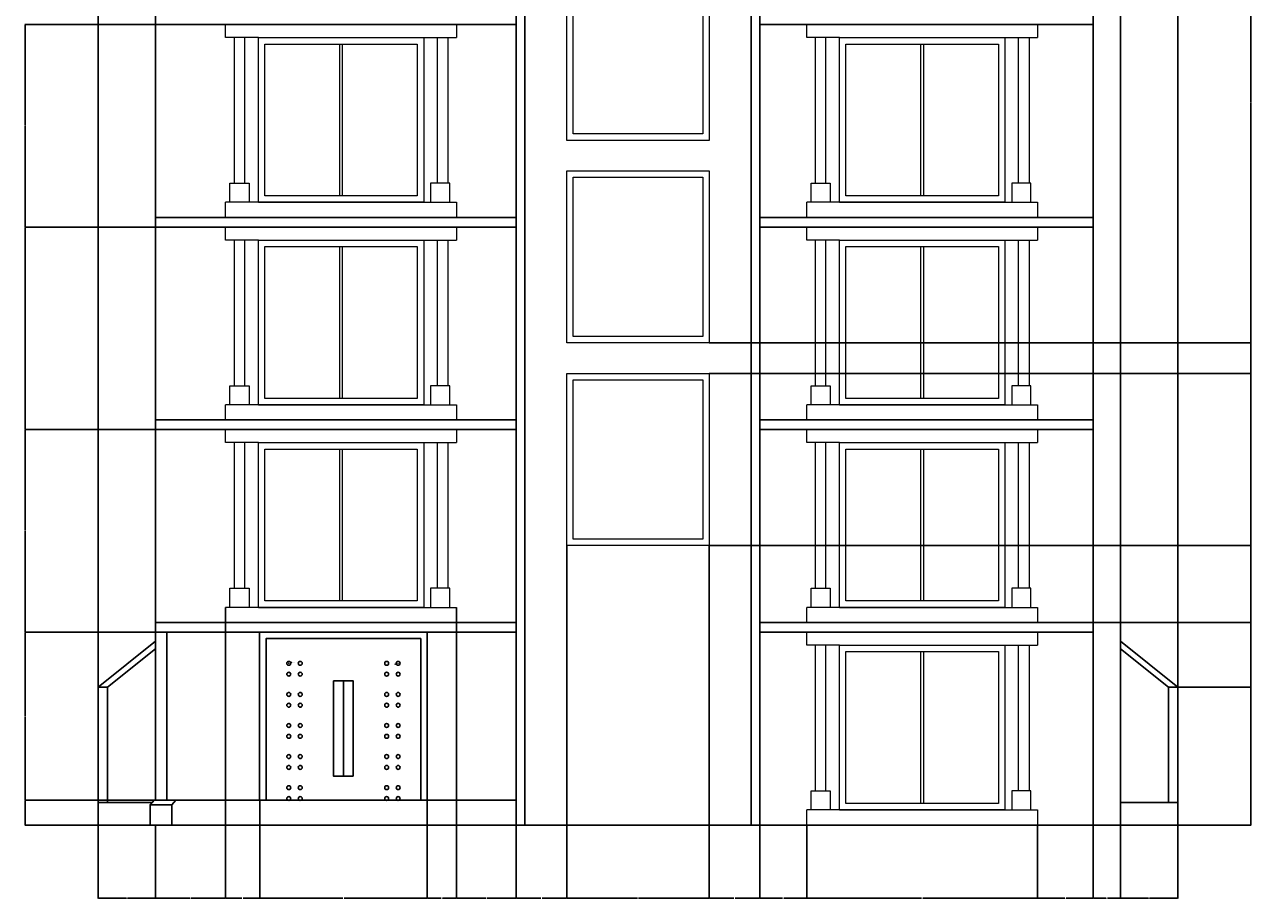
# Model space of a CAD drawing. Units: inches. Extents: x 3024 to 4744, y 1110 to 2100.
# Tile 28 of 29: x 3980 to 4744, y 1110 to 1654. Entities that reach past the tile are written whole.
import ezdxf

# ---------------------------------------------------------------- set-up
doc = ezdxf.new("R2010")
doc.units = ezdxf.units.IN
for name, color, linetype, lineweight in [('A-ANNO-DIMS', 2, 'Continuous', 18), ('A-ELEV', 7, 'Continuous', 25), ('A-GLAZ', 4, 'Continuous', 18)]:
    doc.layers.add(name, color=color, linetype=linetype, lineweight=lineweight)
doc.styles.get("Standard").update_dxf_attribs({"font": 'arial.ttf'})
doc.dimstyles.get("Standard").update_dxf_attribs({"dimtxt": 0.18, "dimasz": 0.18, "dimexe": 0.18, "dimexo": 0.0625, "dimgap": 0.09, "dimtad": 0, "dimtih": 1, "dimtoh": 1, "dimdec": 1, "dimzin": 0, "dimdsep": 46, "dimlunit": 3, "dimtxsty": 'Standard', "dimcen": 0.09, "dimadec": 0, "dimazin": 0, "dimtfac": 1, "dimtdec": 1, "dimtofl": 0, "dimtmove": 0, "dimatfit": 3, "dimfxl": 1, "dimtolj": 1, "dimtzin": 0, "dimarcsym": 0})

# ---------------------------------------------------------------- blocks, each defined once
blk = doc.blocks.new('WIN-BALCONY-B')
for p, q in [((4125.9, 1897.49), (4105.47, 1897.49)), ((4125.9, 1897.49), (4249.1, 1897.49)), ((4125.9, 1795.04), (4105.47, 1795.04)), ((4125.9, 1795.04), (4249.1, 1795.04))]:
    blk.add_line(p, q)
for points in [[(4105.47, 1897.49), (4105.47, 1905.61), (4249.1, 1905.61), (4249.1, 1897.49)], [(4249.1, 1795.04), (4249.1, 1785.61), (4105.47, 1785.61), (4105.47, 1795.04)]]:
    blk.add_lwpolyline(points)
for points in [[(4110.83, 1806.87), (4117.36, 1806.87), (4117.36, 1897.49), (4110.83, 1897.49)], [(4228.68, 1795.04), (4125.9, 1795.04), (4125.9, 1897.49), (4228.68, 1897.49)], [(4224.68, 1799.04), (4129.9, 1799.04), (4129.9, 1893.49), (4224.68, 1893.49)], [(4176.55, 1893.49), (4178.02, 1893.49), (4178.02, 1799.04), (4176.55, 1799.04)], [(4243.74, 1806.87), (4237.21, 1806.87), (4237.21, 1897.49), (4243.74, 1897.49)], [(4120.03, 1795.04), (4108.16, 1795.04), (4108.16, 1806.87), (4120.03, 1806.87)], [(4233.01, 1795.04), (4244.87, 1795.04), (4244.87, 1806.87), (4233.01, 1806.87)]]:
    blk.add_lwpolyline(points, close=True)
blk = doc.blocks.new('WIN-CENTRE-PLAIN')
for points in [[(4317.72, 1940.61), (4406.22, 1940.61), (4406.22, 1833.52), (4317.72, 1833.52)], [(4321.72, 1936.61), (4402.22, 1936.61), (4402.22, 1837.52), (4321.72, 1837.52)]]:
    blk.add_lwpolyline(points, close=True)
blk = doc.blocks.new('*D16')
at = {"layer": 'A-ANNO-DIMS', "color": 0, "lineweight": -2, "transparency": 16777216}
for p, q in [((4026.29, 1155.55), (4026.29, 1109.93)), ((4061.97, 1155.55), (4061.97, 1109.93)), ((4026.47, 1110.11), (4043.74, 1110.11)), ((4061.79, 1110.11), (4044.53, 1110.11))]:
    blk.add_line(p, q, dxfattribs=at)
at = {"layer": 'A-ANNO-DIMS', "color": 0, "transparency": 16777216}
for points in [[(4026.47, 1110.14), (4026.47, 1110.08), (4026.29, 1110.11)], [(4061.79, 1110.14), (4061.79, 1110.08), (4061.97, 1110.11)]]:
    blk.add_solid(points, dxfattribs=at)
at = {"layer": 'Defpoints', "color": 0, "transparency": 16777216}
for p in [(4026.29, 1155.61), (4061.97, 1155.61), (4061.97, 1110.11)]:
    blk.add_point(p, dxfattribs=at)
at = {"layer": 'A-ANNO-DIMS', "color": 0, "transparency": 16777216, "insert": (4044.13, 1110.11), "char_height": 0.18, "attachment_point": 5}
blk.add_mtext('\\A1;35.68', dxfattribs=at)
blk = doc.blocks.new('*D17')
at = {"layer": 'A-ANNO-DIMS', "color": 0, "lineweight": -2, "transparency": 16777216}
for p, q in [((4105.47, 1290.98), (4105.47, 1109.93)), ((4061.97, 1155.55), (4061.97, 1109.93)), ((4062.15, 1110.11), (4083.39, 1110.11)), ((4105.29, 1110.11), (4084.05, 1110.11))]:
    blk.add_line(p, q, dxfattribs=at)
at = {"layer": 'A-ANNO-DIMS', "color": 0, "transparency": 16777216}
for points in [[(4062.15, 1110.14), (4062.15, 1110.08), (4061.97, 1110.11)], [(4105.29, 1110.14), (4105.29, 1110.08), (4105.47, 1110.11)]]:
    blk.add_solid(points, dxfattribs=at)
at = {"layer": 'Defpoints', "color": 0, "transparency": 16777216}
for p in [(4105.47, 1291.04), (4061.97, 1155.61), (4105.47, 1110.11)]:
    blk.add_point(p, dxfattribs=at)
at = {"layer": 'A-ANNO-DIMS', "color": 0, "transparency": 16777216, "insert": (4083.72, 1110.11), "char_height": 0.18, "attachment_point": 5}
blk.add_mtext('\\A1;43.5', dxfattribs=at)
blk = doc.blocks.new('*D18')
at = {"layer": 'A-ANNO-DIMS', "color": 0, "lineweight": -2, "transparency": 16777216}
for p, q in [((4105.47, 1290.98), (4105.47, 1109.93)), ((4126.66, 1170.96), (4126.66, 1109.93)), ((4105.65, 1110.11), (4115.67, 1110.11)), ((4126.48, 1110.11), (4116.46, 1110.11))]:
    blk.add_line(p, q, dxfattribs=at)
at = {"layer": 'A-ANNO-DIMS', "color": 0, "transparency": 16777216}
for points in [[(4105.65, 1110.14), (4105.65, 1110.08), (4105.47, 1110.11)], [(4126.48, 1110.14), (4126.48, 1110.08), (4126.66, 1110.11)]]:
    blk.add_solid(points, dxfattribs=at)
at = {"layer": 'Defpoints', "color": 0, "transparency": 16777216}
for p in [(4105.47, 1291.04), (4126.66, 1171.02), (4126.66, 1110.11)]:
    blk.add_point(p, dxfattribs=at)
at = {"layer": 'A-ANNO-DIMS', "color": 0, "transparency": 16777216, "insert": (4116.06, 1110.11), "char_height": 0.18, "attachment_point": 5}
blk.add_mtext('\\A1;21.19', dxfattribs=at)
blk = doc.blocks.new('*D19')
at = {"layer": 'A-ANNO-DIMS', "color": 0, "lineweight": -2, "transparency": 16777216}
for p, q in [((4126.66, 1170.96), (4126.66, 1109.93)), ((4230.89, 1170.96), (4230.89, 1109.93)), ((4126.84, 1110.11), (4178.32, 1110.11)), ((4230.71, 1110.11), (4179.23, 1110.11))]:
    blk.add_line(p, q, dxfattribs=at)
at = {"layer": 'A-ANNO-DIMS', "color": 0, "transparency": 16777216}
for points in [[(4126.84, 1110.14), (4126.84, 1110.08), (4126.66, 1110.11)], [(4230.71, 1110.14), (4230.71, 1110.08), (4230.89, 1110.11)]]:
    blk.add_solid(points, dxfattribs=at)
at = {"layer": 'Defpoints', "color": 0, "transparency": 16777216}
for p in [(4126.66, 1171.02), (4230.89, 1171.02), (4230.89, 1110.11)]:
    blk.add_point(p, dxfattribs=at)
at = {"layer": 'A-ANNO-DIMS', "color": 0, "transparency": 16777216, "insert": (4178.77, 1110.11), "char_height": 0.18, "attachment_point": 5}
blk.add_mtext('\\A1;104.23', dxfattribs=at)
blk = doc.blocks.new('*D20')
at = {"layer": 'A-ANNO-DIMS', "color": 0, "lineweight": -2, "transparency": 16777216}
for p, q in [((4249.1, 1290.98), (4249.1, 1109.93)), ((4230.89, 1170.96), (4230.89, 1109.93)), ((4231.07, 1110.11), (4239.54, 1110.11)), ((4248.92, 1110.11), (4240.45, 1110.11))]:
    blk.add_line(p, q, dxfattribs=at)
at = {"layer": 'A-ANNO-DIMS', "color": 0, "transparency": 16777216}
for points in [[(4231.07, 1110.14), (4231.07, 1110.08), (4230.89, 1110.11)], [(4248.92, 1110.14), (4248.92, 1110.08), (4249.1, 1110.11)]]:
    blk.add_solid(points, dxfattribs=at)
at = {"layer": 'Defpoints', "color": 0, "transparency": 16777216}
for p in [(4249.1, 1291.04), (4230.89, 1171.02), (4249.1, 1110.11)]:
    blk.add_point(p, dxfattribs=at)
at = {"layer": 'A-ANNO-DIMS', "color": 0, "transparency": 16777216, "insert": (4240, 1110.11), "char_height": 0.18, "attachment_point": 5}
blk.add_mtext('\\A1;18.217', dxfattribs=at)
blk = doc.blocks.new('*D21')
at = {"layer": 'A-ANNO-DIMS', "color": 0, "lineweight": -2, "transparency": 16777216}
for p, q in [((4249.1, 1290.98), (4249.1, 1109.93)), ((4286.2, 1155.55), (4286.2, 1109.93)), ((4249.28, 1110.11), (4267.35, 1110.11)), ((4286.02, 1110.11), (4267.96, 1110.11))]:
    blk.add_line(p, q, dxfattribs=at)
at = {"layer": 'A-ANNO-DIMS', "color": 0, "transparency": 16777216}
for points in [[(4249.28, 1110.14), (4249.28, 1110.08), (4249.1, 1110.11)], [(4286.02, 1110.14), (4286.02, 1110.08), (4286.2, 1110.11)]]:
    blk.add_solid(points, dxfattribs=at)
at = {"layer": 'Defpoints', "color": 0, "transparency": 16777216}
for p in [(4249.1, 1291.04), (4286.2, 1155.61), (4286.2, 1110.11)]:
    blk.add_point(p, dxfattribs=at)
at = {"layer": 'A-ANNO-DIMS', "color": 0, "transparency": 16777216, "insert": (4267.65, 1110.11), "char_height": 0.18, "attachment_point": 5}
blk.add_mtext('\\A1;37.1', dxfattribs=at)
blk = doc.blocks.new('*D22')
at = {"layer": 'A-ANNO-DIMS', "color": 0, "lineweight": -2, "transparency": 16777216}
for p, q in [((4317.72, 1329.46), (4317.72, 1109.93)), ((4286.2, 1155.55), (4286.2, 1109.93)), ((4286.38, 1110.11), (4301.57, 1110.11)), ((4317.54, 1110.11), (4302.36, 1110.11))]:
    blk.add_line(p, q, dxfattribs=at)
at = {"layer": 'A-ANNO-DIMS', "color": 0, "transparency": 16777216}
for points in [[(4286.38, 1110.14), (4286.38, 1110.08), (4286.2, 1110.11)], [(4317.54, 1110.14), (4317.54, 1110.08), (4317.72, 1110.11)]]:
    blk.add_solid(points, dxfattribs=at)
at = {"layer": 'Defpoints', "color": 0, "transparency": 16777216}
for p in [(4317.72, 1329.52), (4286.2, 1155.61), (4317.72, 1110.11)]:
    blk.add_point(p, dxfattribs=at)
at = {"layer": 'A-ANNO-DIMS', "color": 0, "transparency": 16777216, "insert": (4301.96, 1110.11), "char_height": 0.18, "attachment_point": 5}
blk.add_mtext('\\A1;31.52', dxfattribs=at)
blk = doc.blocks.new('*D23')
at = {"layer": 'A-ANNO-DIMS', "color": 0, "lineweight": -2, "transparency": 16777216}
for p, q in [((4317.72, 1329.46), (4317.72, 1109.93)), ((4406.22, 1329.46), (4406.22, 1109.93)), ((4317.9, 1110.11), (4361.65, 1110.11)), ((4406.04, 1110.11), (4362.3, 1110.11))]:
    blk.add_line(p, q, dxfattribs=at)
at = {"layer": 'A-ANNO-DIMS', "color": 0, "transparency": 16777216}
for points in [[(4317.9, 1110.14), (4317.9, 1110.08), (4317.72, 1110.11)], [(4406.04, 1110.14), (4406.04, 1110.08), (4406.22, 1110.11)]]:
    blk.add_solid(points, dxfattribs=at)
at = {"layer": 'Defpoints', "color": 0, "transparency": 16777216}
for p in [(4317.72, 1329.52), (4406.22, 1329.52), (4406.22, 1110.11)]:
    blk.add_point(p, dxfattribs=at)
at = {"layer": 'A-ANNO-DIMS', "color": 0, "transparency": 16777216, "insert": (4361.97, 1110.11), "char_height": 0.18, "attachment_point": 5}
blk.add_mtext('\\A1;88.5', dxfattribs=at)
blk = doc.blocks.new('*D24')
at = {"layer": 'A-ANNO-DIMS', "color": 0, "lineweight": -2, "transparency": 16777216}
for p, q in [((4406.22, 1329.46), (4406.22, 1109.93)), ((4437.74, 1155.55), (4437.74, 1109.93)), ((4406.4, 1110.11), (4421.59, 1110.11)), ((4437.56, 1110.11), (4422.37, 1110.11))]:
    blk.add_line(p, q, dxfattribs=at)
at = {"layer": 'A-ANNO-DIMS', "color": 0, "transparency": 16777216}
for points in [[(4406.4, 1110.14), (4406.4, 1110.08), (4406.22, 1110.11)], [(4437.56, 1110.14), (4437.56, 1110.08), (4437.74, 1110.11)]]:
    blk.add_solid(points, dxfattribs=at)
at = {"layer": 'Defpoints', "color": 0, "transparency": 16777216}
for p in [(4406.22, 1329.52), (4437.74, 1155.61), (4437.74, 1110.11)]:
    blk.add_point(p, dxfattribs=at)
at = {"layer": 'A-ANNO-DIMS', "color": 0, "transparency": 16777216, "insert": (4421.98, 1110.11), "char_height": 0.18, "attachment_point": 5}
blk.add_mtext('\\A1;31.52', dxfattribs=at)
blk = doc.blocks.new('*D25')
at = {"layer": 'A-ANNO-DIMS', "color": 0, "lineweight": -2, "transparency": 16777216}
for p, q in [((4437.74, 1155.55), (4437.74, 1109.93)), ((4466.9, 1155.55), (4466.9, 1109.93)), ((4437.92, 1110.11), (4451.92, 1110.11)), ((4466.72, 1110.11), (4452.72, 1110.11))]:
    blk.add_line(p, q, dxfattribs=at)
at = {"layer": 'A-ANNO-DIMS', "color": 0, "transparency": 16777216}
for points in [[(4437.92, 1110.14), (4437.92, 1110.08), (4437.74, 1110.11)], [(4466.72, 1110.14), (4466.72, 1110.08), (4466.9, 1110.11)]]:
    blk.add_solid(points, dxfattribs=at)
at = {"layer": 'Defpoints', "color": 0, "transparency": 16777216}
for p in [(4437.74, 1155.61), (4466.9, 1155.61), (4466.9, 1110.11)]:
    blk.add_point(p, dxfattribs=at)
at = {"layer": 'A-ANNO-DIMS', "color": 0, "transparency": 16777216, "insert": (4452.32, 1110.11), "char_height": 0.18, "attachment_point": 5}
blk.add_mtext('\\A1;29.16', dxfattribs=at)
blk = doc.blocks.new('*D26')
at = {"layer": 'A-ANNO-DIMS', "color": 0, "lineweight": -2, "transparency": 16777216}
for p, q in [((4466.9, 1155.55), (4466.9, 1109.93)), ((4610.54, 1155.55), (4610.54, 1109.93)), ((4467.08, 1110.11), (4538.26, 1110.11)), ((4610.36, 1110.11), (4539.17, 1110.11))]:
    blk.add_line(p, q, dxfattribs=at)
at = {"layer": 'A-ANNO-DIMS', "color": 0, "transparency": 16777216}
for points in [[(4467.08, 1110.14), (4467.08, 1110.08), (4466.9, 1110.11)], [(4610.36, 1110.14), (4610.36, 1110.08), (4610.54, 1110.11)]]:
    blk.add_solid(points, dxfattribs=at)
at = {"layer": 'Defpoints', "color": 0, "transparency": 16777216}
for p in [(4466.9, 1155.61), (4610.54, 1155.61), (4610.54, 1110.11)]:
    blk.add_point(p, dxfattribs=at)
at = {"layer": 'A-ANNO-DIMS', "color": 0, "transparency": 16777216, "insert": (4538.72, 1110.11), "char_height": 0.18, "attachment_point": 5}
blk.add_mtext('\\A1;143.64', dxfattribs=at)
blk = doc.blocks.new('*D27')
at = {"layer": 'A-ANNO-DIMS', "color": 0, "lineweight": -2, "transparency": 16777216}
for p, q in [((4610.54, 1155.55), (4610.54, 1109.93)), ((4645.06, 1155.55), (4645.06, 1109.93)), ((4610.72, 1110.11), (4627.4, 1110.11)), ((4644.88, 1110.11), (4628.19, 1110.11))]:
    blk.add_line(p, q, dxfattribs=at)
at = {"layer": 'A-ANNO-DIMS', "color": 0, "transparency": 16777216}
for points in [[(4610.72, 1110.14), (4610.72, 1110.08), (4610.54, 1110.11)], [(4644.88, 1110.14), (4644.88, 1110.08), (4645.06, 1110.11)]]:
    blk.add_solid(points, dxfattribs=at)
at = {"layer": 'Defpoints', "color": 0, "transparency": 16777216}
for p in [(4610.54, 1155.61), (4645.06, 1155.61), (4645.06, 1110.11)]:
    blk.add_point(p, dxfattribs=at)
at = {"layer": 'A-ANNO-DIMS', "color": 0, "transparency": 16777216, "insert": (4627.8, 1110.11), "char_height": 0.18, "attachment_point": 5}
blk.add_mtext('\\A1;34.52', dxfattribs=at)
blk = doc.blocks.new('*D28')
at = {"layer": 'A-ANNO-DIMS', "color": 0, "lineweight": -2, "transparency": 16777216}
for p, q in [((4645.06, 1155.55), (4645.06, 1109.93)), ((4661.97, 1155.55), (4661.97, 1109.93)), ((4645.24, 1110.11), (4653.06, 1110.11)), ((4661.79, 1110.11), (4653.97, 1110.11))]:
    blk.add_line(p, q, dxfattribs=at)
at = {"layer": 'A-ANNO-DIMS', "color": 0, "transparency": 16777216}
for points in [[(4645.24, 1110.14), (4645.24, 1110.08), (4645.06, 1110.11)], [(4661.79, 1110.14), (4661.79, 1110.08), (4661.97, 1110.11)]]:
    blk.add_solid(points, dxfattribs=at)
at = {"layer": 'Defpoints', "color": 0, "transparency": 16777216}
for p in [(4645.06, 1155.61), (4661.97, 1155.61), (4661.97, 1110.11)]:
    blk.add_point(p, dxfattribs=at)
at = {"layer": 'A-ANNO-DIMS', "color": 0, "transparency": 16777216, "insert": (4653.51, 1110.11), "char_height": 0.18, "attachment_point": 5}
blk.add_mtext('\\A1;16.913', dxfattribs=at)
blk = doc.blocks.new('*D29')
at = {"layer": 'A-ANNO-DIMS', "color": 0, "lineweight": -2, "transparency": 16777216}
for p, q in [((4661.97, 1155.55), (4661.97, 1109.93)), ((4697.65, 1155.55), (4697.65, 1109.93)), ((4662.15, 1110.11), (4679.42, 1110.11)), ((4697.47, 1110.11), (4680.2, 1110.11))]:
    blk.add_line(p, q, dxfattribs=at)
at = {"layer": 'A-ANNO-DIMS', "color": 0, "transparency": 16777216}
for points in [[(4662.15, 1110.14), (4662.15, 1110.08), (4661.97, 1110.11)], [(4697.47, 1110.14), (4697.47, 1110.08), (4697.65, 1110.11)]]:
    blk.add_solid(points, dxfattribs=at)
at = {"layer": 'Defpoints', "color": 0, "transparency": 16777216}
for p in [(4661.97, 1155.61), (4697.65, 1155.61), (4697.65, 1110.11)]:
    blk.add_point(p, dxfattribs=at)
at = {"layer": 'A-ANNO-DIMS', "color": 0, "transparency": 16777216, "insert": (4679.81, 1110.11), "char_height": 0.18, "attachment_point": 5}
blk.add_mtext('\\A1;35.68', dxfattribs=at)
blk = doc.blocks.new('*D30')
at = {"layer": 'A-ANNO-DIMS', "color": 0, "lineweight": -2, "transparency": 16777216}
for p, q in [((4026.29, 1241.5), (4026.29, 2100.44)), ((4026.47, 2100.26), (4038.86, 2100.26)), ((4052.03, 2100.26), (4039.65, 2100.26)), ((4052.21, 1911.67), (4052.21, 2100.44))]:
    blk.add_line(p, q, dxfattribs=at)
at = {"layer": 'A-ANNO-DIMS', "color": 0, "transparency": 16777216}
for points in [[(4026.47, 2100.29), (4026.47, 2100.23), (4026.29, 2100.26)], [(4052.03, 2100.29), (4052.03, 2100.23), (4052.21, 2100.26)]]:
    blk.add_solid(points, dxfattribs=at)
at = {"layer": 'Defpoints', "color": 0, "transparency": 16777216}
for p in [(4052.21, 2100.26), (4052.21, 1911.61), (4026.29, 1241.43)]:
    blk.add_point(p, dxfattribs=at)
at = {"layer": 'A-ANNO-DIMS', "color": 0, "transparency": 16777216, "insert": (4039.25, 2100.26), "char_height": 0.18, "attachment_point": 5}
blk.add_mtext('\\A1;25.92', dxfattribs=at)
blk = doc.blocks.new('*D34')
at = {"layer": 'A-ANNO-DIMS', "color": 0, "lineweight": -2, "transparency": 16777216}
for p, q in [((4671.73, 1911.67), (4671.73, 2100.44)), ((4671.91, 2100.26), (4684.29, 2100.26)), ((4697.47, 2100.26), (4685.08, 2100.26)), ((4697.65, 1241.5), (4697.65, 2100.44))]:
    blk.add_line(p, q, dxfattribs=at)
at = {"layer": 'A-ANNO-DIMS', "color": 0, "transparency": 16777216}
for points in [[(4671.91, 2100.29), (4671.91, 2100.23), (4671.73, 2100.26)], [(4697.47, 2100.29), (4697.47, 2100.23), (4697.65, 2100.26)]]:
    blk.add_solid(points, dxfattribs=at)
at = {"layer": 'Defpoints', "color": 0, "transparency": 16777216}
for p in [(4697.65, 2100.26), (4671.73, 1911.61), (4697.65, 1241.43)]:
    blk.add_point(p, dxfattribs=at)
at = {"layer": 'A-ANNO-DIMS', "color": 0, "transparency": 16777216, "insert": (4684.69, 2100.26), "char_height": 0.18, "attachment_point": 5}
blk.add_mtext('\\A1;25.92', dxfattribs=at)
blk = doc.blocks.new('*D35')
at = {"layer": 'A-ANNO-DIMS', "color": 0, "lineweight": -2, "transparency": 16777216}
for p, q in [((4061.91, 1171.02), (3980.61, 1171.02)), ((3980.79, 1170.84), (3980.79, 1163.5)), ((3980.79, 1155.79), (3980.79, 1163.14)), ((4061.91, 1155.61), (3980.61, 1155.61))]:
    blk.add_line(p, q, dxfattribs=at)
at = {"layer": 'A-ANNO-DIMS', "color": 0, "transparency": 16777216}
for points in [[(3980.76, 1170.84), (3980.82, 1170.84), (3980.79, 1171.02)], [(3980.76, 1155.79), (3980.82, 1155.79), (3980.79, 1155.61)]]:
    blk.add_solid(points, dxfattribs=at)
at = {"layer": 'Defpoints', "color": 0, "transparency": 16777216}
for p in [(3980.79, 1171.02), (4061.97, 1171.02), (4061.97, 1155.61)]:
    blk.add_point(p, dxfattribs=at)
at = {"layer": 'A-ANNO-DIMS', "color": 0, "transparency": 16777216, "insert": (3980.79, 1163.32), "char_height": 0.18, "attachment_point": 5}
blk.add_mtext('\\A1;15.413', dxfattribs=at)
blk = doc.blocks.new('*D36')
at = {"layer": 'A-ANNO-DIMS', "color": 0, "lineweight": -2, "transparency": 16777216}
for p, q in [((4061.91, 1275.61), (3980.61, 1275.61)), ((3980.79, 1275.43), (3980.79, 1223.5)), ((3980.79, 1171.2), (3980.79, 1223.14)), ((4061.91, 1171.02), (3980.61, 1171.02))]:
    blk.add_line(p, q, dxfattribs=at)
at = {"layer": 'A-ANNO-DIMS', "color": 0, "transparency": 16777216}
for points in [[(3980.76, 1275.43), (3980.82, 1275.43), (3980.79, 1275.61)], [(3980.76, 1171.2), (3980.82, 1171.2), (3980.79, 1171.02)]]:
    blk.add_solid(points, dxfattribs=at)
at = {"layer": 'Defpoints', "color": 0, "transparency": 16777216}
for p in [(3980.79, 1275.61), (4061.97, 1275.61), (4061.97, 1171.02)]:
    blk.add_point(p, dxfattribs=at)
at = {"layer": 'A-ANNO-DIMS', "color": 0, "transparency": 16777216, "insert": (3980.79, 1223.32), "char_height": 0.18, "attachment_point": 5}
blk.add_mtext('\\A1;104.59', dxfattribs=at)
blk = doc.blocks.new('*D37')
at = {"layer": 'A-ANNO-DIMS', "color": 0, "lineweight": -2, "transparency": 16777216}
for p, q in [((4061.91, 1401.61), (3980.61, 1401.61)), ((3980.79, 1401.43), (3980.79, 1338.79)), ((3980.79, 1275.79), (3980.79, 1338.43)), ((4061.91, 1275.61), (3980.61, 1275.61))]:
    blk.add_line(p, q, dxfattribs=at)
at = {"layer": 'A-ANNO-DIMS', "color": 0, "transparency": 16777216}
for points in [[(3980.76, 1401.43), (3980.82, 1401.43), (3980.79, 1401.61)], [(3980.76, 1275.79), (3980.82, 1275.79), (3980.79, 1275.61)]]:
    blk.add_solid(points, dxfattribs=at)
at = {"layer": 'Defpoints', "color": 0, "transparency": 16777216}
for p in [(3980.79, 1401.61), (4061.97, 1401.61), (4061.97, 1275.61)]:
    blk.add_point(p, dxfattribs=at)
at = {"layer": 'A-ANNO-DIMS', "color": 0, "transparency": 16777216, "insert": (3980.79, 1338.61), "char_height": 0.18, "attachment_point": 5}
blk.add_mtext('\\A1;126', dxfattribs=at)
blk = doc.blocks.new('*D38')
at = {"layer": 'A-ANNO-DIMS', "color": 0, "lineweight": -2, "transparency": 16777216}
for p, q in [((4061.91, 1527.61), (3980.61, 1527.61)), ((3980.79, 1527.43), (3980.79, 1464.79)), ((3980.79, 1401.79), (3980.79, 1464.43)), ((4061.91, 1401.61), (3980.61, 1401.61))]:
    blk.add_line(p, q, dxfattribs=at)
at = {"layer": 'A-ANNO-DIMS', "color": 0, "transparency": 16777216}
for points in [[(3980.76, 1527.43), (3980.82, 1527.43), (3980.79, 1527.61)], [(3980.76, 1401.79), (3980.82, 1401.79), (3980.79, 1401.61)]]:
    blk.add_solid(points, dxfattribs=at)
at = {"layer": 'Defpoints', "color": 0, "transparency": 16777216}
for p in [(3980.79, 1527.61), (4061.97, 1527.61), (4061.97, 1401.61)]:
    blk.add_point(p, dxfattribs=at)
at = {"layer": 'A-ANNO-DIMS', "color": 0, "transparency": 16777216, "insert": (3980.79, 1464.61), "char_height": 0.18, "attachment_point": 5}
blk.add_mtext('\\A1;126', dxfattribs=at)
blk = doc.blocks.new('*D39')
at = {"layer": 'A-ANNO-DIMS', "color": 0, "lineweight": -2, "transparency": 16777216}
for p, q in [((4061.91, 1653.61), (3980.61, 1653.61)), ((3980.79, 1653.43), (3980.79, 1590.79)), ((3980.79, 1527.79), (3980.79, 1590.43)), ((4061.91, 1527.61), (3980.61, 1527.61))]:
    blk.add_line(p, q, dxfattribs=at)
at = {"layer": 'A-ANNO-DIMS', "color": 0, "transparency": 16777216}
for points in [[(3980.76, 1653.43), (3980.82, 1653.43), (3980.79, 1653.61)], [(3980.76, 1527.79), (3980.82, 1527.79), (3980.79, 1527.61)]]:
    blk.add_solid(points, dxfattribs=at)
at = {"layer": 'Defpoints', "color": 0, "transparency": 16777216}
for p in [(3980.79, 1653.61), (4061.97, 1653.61), (4061.97, 1527.61)]:
    blk.add_point(p, dxfattribs=at)
at = {"layer": 'A-ANNO-DIMS', "color": 0, "transparency": 16777216, "insert": (3980.79, 1590.61), "char_height": 0.18, "attachment_point": 5}
blk.add_mtext('\\A1;126', dxfattribs=at)
blk = doc.blocks.new('*D45')
at = {"layer": 'A-ANNO-DIMS', "color": 0, "lineweight": -2, "transparency": 16777216}
for p, q in [((4697.71, 1241.43), (4743.33, 1241.43)), ((4743.15, 1241.25), (4743.15, 1198.7)), ((4743.15, 1155.79), (4743.15, 1198.34)), ((4697.71, 1155.61), (4743.33, 1155.61))]:
    blk.add_line(p, q, dxfattribs=at)
at = {"layer": 'A-ANNO-DIMS', "color": 0, "transparency": 16777216}
for points in [[(4743.12, 1241.25), (4743.18, 1241.25), (4743.15, 1241.43)], [(4743.12, 1155.79), (4743.18, 1155.79), (4743.15, 1155.61)]]:
    blk.add_solid(points, dxfattribs=at)
at = {"layer": 'Defpoints', "color": 0, "transparency": 16777216}
for p in [(4697.65, 1241.43), (4743.15, 1241.43), (4697.65, 1155.61)]:
    blk.add_point(p, dxfattribs=at)
at = {"layer": 'A-ANNO-DIMS', "color": 0, "transparency": 16777216, "insert": (4743.15, 1198.52), "char_height": 0.18, "attachment_point": 5}
blk.add_mtext('\\A1;85.82', dxfattribs=at)
blk = doc.blocks.new('*D46')
at = {"layer": 'A-ANNO-DIMS', "color": 0, "lineweight": -2, "transparency": 16777216}
for p, q in [((4406.28, 1329.52), (4743.33, 1329.52)), ((4743.15, 1329.34), (4743.15, 1305.75)), ((4743.15, 1281.79), (4743.15, 1305.39)), ((4645.12, 1281.61), (4743.33, 1281.61))]:
    blk.add_line(p, q, dxfattribs=at)
at = {"layer": 'A-ANNO-DIMS', "color": 0, "transparency": 16777216}
for points in [[(4743.12, 1329.34), (4743.18, 1329.34), (4743.15, 1329.52)], [(4743.12, 1281.79), (4743.18, 1281.79), (4743.15, 1281.61)]]:
    blk.add_solid(points, dxfattribs=at)
at = {"layer": 'Defpoints', "color": 0, "transparency": 16777216}
for p in [(4406.22, 1329.52), (4743.15, 1329.52), (4645.06, 1281.61)]:
    blk.add_point(p, dxfattribs=at)
at = {"layer": 'A-ANNO-DIMS', "color": 0, "transparency": 16777216, "insert": (4743.15, 1305.57), "char_height": 0.18, "attachment_point": 5}
blk.add_mtext('\\A1;47.91', dxfattribs=at)
blk = doc.blocks.new('*D47')
at = {"layer": 'A-ANNO-DIMS', "color": 0, "lineweight": -2, "transparency": 16777216}
for p, q in [((4406.28, 1455.52), (4743.33, 1455.52)), ((4743.15, 1455.34), (4743.15, 1446.25)), ((4743.15, 1436.79), (4743.15, 1445.88)), ((4406.28, 1436.61), (4743.33, 1436.61))]:
    blk.add_line(p, q, dxfattribs=at)
at = {"layer": 'A-ANNO-DIMS', "color": 0, "transparency": 16777216}
for points in [[(4743.12, 1455.34), (4743.18, 1455.34), (4743.15, 1455.52)], [(4743.12, 1436.79), (4743.18, 1436.79), (4743.15, 1436.61)]]:
    blk.add_solid(points, dxfattribs=at)
at = {"layer": 'Defpoints', "color": 0, "transparency": 16777216}
for p in [(4406.22, 1455.52), (4743.15, 1455.52), (4406.22, 1436.61)]:
    blk.add_point(p, dxfattribs=at)
at = {"layer": 'A-ANNO-DIMS', "color": 0, "transparency": 16777216, "insert": (4743.15, 1446.07), "char_height": 0.18, "attachment_point": 5}
blk.add_mtext('\\A1;18.92', dxfattribs=at)
blk = doc.blocks.new('*D76')
at = {"layer": 'A-ANNO-DIMS', "color": 0, "lineweight": -2, "transparency": 16777216}
for p, q in [((4144.67, 1256.23), (4144.85, 1256.23)), ((4144.76, 1256.14), (4144.76, 1256.32)), ((4146.57, 1256.89), (4146.06, 1256.71)), ((4146.75, 1256.89), (4146.57, 1256.89))]:
    blk.add_line(p, q, dxfattribs=at)
at = {"layer": 'A-ANNO-DIMS', "color": 0, "transparency": 16777216}
blk.add_solid([(4146.05, 1256.73), (4146.07, 1256.68), (4145.89, 1256.64)], dxfattribs=at)
at = {"layer": 'Defpoints', "color": 0, "transparency": 16777216}
for p in [(4143.62, 1255.81), (4145.89, 1256.64)]:
    blk.add_point(p, dxfattribs=at)
at = {"layer": 'A-ANNO-DIMS', "color": 0, "transparency": 16777216, "insert": (4147.5, 1256.89), "char_height": 0.18, "attachment_point": 5}
blk.add_mtext('\\A1;40X ∅2.414', dxfattribs=at)
blk = doc.blocks.new('*D78')
at = {"layer": 'A-ANNO-DIMS', "color": 0, "lineweight": -2, "transparency": 16777216}
for p, q in [((4448.39, 2054.76), (4743.33, 2054.76)), ((4743.15, 2054.58), (4743.15, 1605.37)), ((4743.15, 1155.79), (4743.15, 1605)), ((4697.71, 1155.61), (4743.33, 1155.61))]:
    blk.add_line(p, q, dxfattribs=at)
at = {"layer": 'A-ANNO-DIMS', "color": 0, "transparency": 16777216}
for points in [[(4743.12, 2054.58), (4743.18, 2054.58), (4743.15, 2054.76)], [(4743.12, 1155.79), (4743.18, 1155.79), (4743.15, 1155.61)]]:
    blk.add_solid(points, dxfattribs=at)
at = {"layer": 'Defpoints', "color": 0, "transparency": 16777216}
for p in [(4448.33, 2054.76), (4743.15, 2054.76), (4697.65, 1155.61)]:
    blk.add_point(p, dxfattribs=at)
at = {"layer": 'A-ANNO-DIMS', "color": 0, "transparency": 16777216, "insert": (4743.15, 1605.18), "char_height": 0.18, "attachment_point": 5}
blk.add_mtext('\\A1;899.15', dxfattribs=at)
blk = doc.blocks.new('*D130')
at = {"layer": 'A-ANNO-DIMS', "color": 0, "lineweight": -2, "transparency": 16777216}
for p, q in [((4210.76, 1255.66), (4210.94, 1255.66)), ((4210.94, 1255.66), (4211.46, 1255.82)), ((4212.7, 1256.23), (4212.88, 1256.23)), ((4212.79, 1256.14), (4212.79, 1256.32))]:
    blk.add_line(p, q, dxfattribs=at)
at = {"layer": 'A-ANNO-DIMS', "color": 0, "transparency": 16777216}
blk.add_solid([(4211.46, 1255.85), (4211.47, 1255.79), (4211.64, 1255.87)], dxfattribs=at)
at = {"layer": 'Defpoints', "color": 0, "transparency": 16777216}
for p in [(4211.64, 1255.87), (4213.94, 1256.59)]:
    blk.add_point(p, dxfattribs=at)
at = {"layer": 'A-ANNO-DIMS', "color": 0, "transparency": 16777216, "insert": (4210.01, 1255.66), "char_height": 0.18, "attachment_point": 5}
blk.add_mtext('\\A1;40X ∅2.414', dxfattribs=at)

msp = doc.modelspace()

# ---------------------------------------------------------------- linework, layer by layer
at = {"layer": 'A-ELEV'}
for p, q in [((4661.9711, 1155.6112), (4661.9711, 1911.6112)), ((4061.9711, 1171.0239), (4061.9711, 1905.6112)), ((4286.2022, 1653.6112), (4061.9711, 1653.6112)), ((4645.0576, 1653.6112), (4437.74, 1653.6112)), ((4061.9711, 1533.6112), (4286.2022, 1533.6112)), ((4286.2022, 1527.6112), (4061.9711, 1527.6112)), ((4437.74, 1533.6112), (4645.0576, 1533.6112)), ((4645.0576, 1527.6112), (4437.74, 1527.6112)), ((4061.9711, 1407.6112), (4286.2022, 1407.6112)), ((4437.74, 1407.6112), (4645.0576, 1407.6112)), ((4286.2022, 1401.6112), (4061.9711, 1401.6112)), ((4645.0576, 1401.6112), (4437.74, 1401.6112)), ((4061.9711, 1275.6112), (4061.9711, 1281.6112)), ((4061.9711, 1281.6112), (4286.2022, 1281.6112)), ((4286.2022, 1275.6112), (4061.9711, 1275.6112)), ((4437.74, 1281.6112), (4645.0576, 1281.6112)), ((4645.0576, 1275.6112), (4437.74, 1275.6112)), ((4026.2926, 1241.4341), (4061.9711, 1269.9091)), ((4697.6496, 1241.4341), (4661.9711, 1269.9091)), ((4032.0358, 1241.4341), (4061.9711, 1265.3254)), ((4691.9063, 1241.4341), (4661.9711, 1265.3254)), ((4178.7732, 1245.2708), (4178.7732, 1185.9515)), ((4026.2926, 1155.6112), (4026.2926, 1169.5534)), ((4059.7347, 1169.5534), (4026.2926, 1169.5534)), ((4058.4636, 1168.0828), (4061.0058, 1171.0239)), ((4058.4636, 1168.0828), (4072.0743, 1168.0828)), ((4061.0058, 1171.0239), (4074.6165, 1171.0239)), ((4072.0743, 1168.0828), (4074.6165, 1171.0239)), ((4074.6165, 1171.0239), (4286.2022, 1171.0239)), ((4661.9711, 1169.5534), (4697.6496, 1169.5534)), ((4697.6496, 1155.6112), (4697.6496, 1169.5534)), ((4061.9711, 1155.6112), (4026.2926, 1155.6112)), ((4061.9711, 1155.6112), (4661.9711, 1155.6112)), ((4661.9711, 1155.6112), (4697.6496, 1155.6112))]:
    msp.add_line(p, q, dxfattribs=at)
for points in [[(4437.74, 1155.6112), (4286.2022, 1155.6112), (4286.2022, 2043.5286), (4437.74, 2043.5286)], [(4286.2022, 2043.5286), (4291.6033, 2043.5286), (4291.6033, 1155.6112), (4286.2022, 1155.6112)], [(4432.3389, 2043.5286), (4437.74, 2043.5286), (4437.74, 1155.6112), (4432.3389, 1155.6112)], [(4184.8844, 1185.9515), (4172.6619, 1185.9515), (4172.6619, 1245.2708), (4184.8844, 1245.2708)], [(4026.2926, 1169.5534), (4032.0358, 1169.5534), (4032.0358, 1241.4341), (4026.2926, 1241.4341)], [(4697.6496, 1169.5534), (4691.9063, 1169.5534), (4691.9063, 1241.4341), (4697.6496, 1241.4341)]]:
    msp.add_lwpolyline(points, close=True, dxfattribs=at)
for points in [[(4661.9711, 1155.6112), (4645.0576, 1155.6112), (4645.0576, 2009.1664)], [(4061.9711, 1275.6112), (4068.8827, 1275.6112), (4068.8827, 1171.0239)], [(4126.6597, 1171.0239), (4126.6597, 1275.6112), (4230.8866, 1275.6112), (4230.8866, 1171.0239)], [(4130.6597, 1171.0239), (4130.6597, 1271.6112), (4226.8866, 1271.6112), (4226.8866, 1171.0239)], [(4072.0743, 1155.6112), (4072.0743, 1168.0828), (4058.4636, 1168.0828), (4058.4636, 1155.6112)], [(4230.8866, 1155.6112), (4126.6597, 1155.6112)]]:
    msp.add_lwpolyline(points, dxfattribs=at)
for centre in [(4144.7575, 1256.2276), (4151.9042, 1256.2276), (4205.6422, 1256.2276), (4212.7888, 1256.2276), (4144.7575, 1249.4899), (4151.9042, 1249.4899), (4205.6422, 1249.4899), (4212.7888, 1249.4899), (4144.7575, 1236.8869), (4151.9042, 1236.8869), (4205.6422, 1236.8869), (4212.7888, 1236.8869), (4144.7575, 1230.1493), (4151.9042, 1230.1493), (4205.6422, 1230.1493), (4212.7888, 1230.1493), (4144.7575, 1217.5463), (4151.9042, 1217.5463), (4205.6422, 1217.5463), (4212.7888, 1217.5463), (4144.7575, 1210.8086), (4151.9042, 1210.8086), (4205.6422, 1210.8086), (4212.7888, 1210.8086), (4144.7575, 1198.2057), (4151.9042, 1198.2057), (4205.6422, 1198.2057), (4212.7888, 1198.2057), (4144.7575, 1191.468), (4151.9042, 1191.468), (4205.6422, 1191.468), (4212.7888, 1191.468), (4144.7575, 1178.8651), (4151.9042, 1178.8651), (4205.6422, 1178.8651), (4212.7888, 1178.8651), (4144.7575, 1172.1274), (4151.9042, 1172.1274), (4205.6422, 1172.1274), (4212.7888, 1172.1274)]:
    msp.add_circle(centre, 1.2071, dxfattribs=at)

# ---------------------------------------------------------------- block references
at = {"layer": 'A-GLAZ'}
for name, p in [('WIN-CENTRE-PLAIN', (0, -252)), ('WIN-BALCONY-B', (0, -252)), ('WIN-BALCONY-B', (361.4319, -252)), ('WIN-CENTRE-PLAIN', (0, -378)), ('WIN-BALCONY-B', (0, -378)), ('WIN-BALCONY-B', (361.4319, -378)), ('WIN-CENTRE-PLAIN', (0, -504)), ('WIN-BALCONY-B', (0, -504)), ('WIN-BALCONY-B', (361.4319, -504)), ('WIN-BALCONY-B', (361.4319, -630))]:
    msp.add_blockref(name, p, dxfattribs=at)

# ---------------------------------------------------------------- dimensions: what is measured, and where the dimension line sits
at = {"layer": 'A-ANNO-DIMS'}
for base, p1, p2, override, picture, middle in [((4052.2147, 2100.2584), (4026.2926, 1241.4341), (4052.2147, 1911.6112), {"dimdec": 2, "dimlfac": 1, "dimrnd": 0, "dimzin": 0, "dimdsep": 46, "dimlunit": 2}, '*D30', (4039.2536, 2100.2584)), ((4697.6496, 2100.2584), (4671.7274, 1911.6112), (4697.6496, 1241.4341), {"dimdec": 2, "dimlfac": 1, "dimrnd": 0, "dimzin": 0, "dimdsep": 46, "dimlunit": 2}, '*D34', (4684.6885, 2100.2584)), ((4317.7231, 1110.1112), (4286.2022, 1155.6112), (4317.7231, 1329.5246), {"dimdec": 2, "dimlfac": 1, "dimrnd": 0, "dimzin": 0, "dimdsep": 46, "dimlunit": 2}, '*D22', (4301.9626, 1110.1112)), ((4406.2191, 1110.1112), (4317.7231, 1329.5246), (4406.2191, 1329.5246), {"dimdec": 1, "dimlfac": 1, "dimrnd": 0, "dimzin": 0, "dimdsep": 46, "dimlunit": 2}, '*D23', (4361.9711, 1110.1112)), ((4437.74, 1110.1112), (4406.2191, 1329.5246), (4437.74, 1155.6112), {"dimdec": 2, "dimlfac": 1, "dimrnd": 0, "dimzin": 0, "dimdsep": 46, "dimlunit": 2}, '*D24', (4421.9795, 1110.1112)), ((4105.4683, 1110.1112), (4061.9711, 1155.6112), (4105.4683, 1291.0431), {"dimdec": 1, "dimlfac": 1, "dimrnd": 0, "dimzin": 0, "dimdsep": 46, "dimlunit": 2}, '*D17', (4083.7197, 1110.1112)), ((4126.6597, 1110.1112), (4105.4683, 1291.0431), (4126.6597, 1171.0239), {"dimdec": 2, "dimlfac": 1, "dimrnd": 0, "dimzin": 0, "dimdsep": 46, "dimlunit": 2}, '*D18', (4116.064, 1110.1112)), ((4249.104, 1110.1112), (4230.8866, 1171.0239), (4249.104, 1291.0431), {"dimdec": 3, "dimlfac": 1, "dimrnd": 0, "dimzin": 0, "dimdsep": 46, "dimlunit": 2}, '*D20', (4239.9953, 1110.1112)), ((4286.2022, 1110.1112), (4249.104, 1291.0431), (4286.2022, 1155.6112), {"dimdec": 1, "dimlfac": 1, "dimrnd": 0, "dimzin": 0, "dimdsep": 46, "dimlunit": 2}, '*D21', (4267.6531, 1110.1112)), ((4230.8866, 1110.1112), (4126.6597, 1171.0239), (4230.8866, 1171.0239), {"dimdec": 2, "dimlfac": 1, "dimrnd": 0, "dimzin": 0, "dimdsep": 46, "dimlunit": 2}, '*D19', (4178.7732, 1110.1112)), ((4061.9711, 1110.1112), (4026.2926, 1155.6112), (4061.9711, 1155.6112), {"dimdec": 2, "dimlfac": 1, "dimrnd": 0, "dimzin": 0, "dimdsep": 46, "dimlunit": 2}, '*D16', (4044.1318, 1110.1112)), ((4466.9002, 1110.1112), (4437.74, 1155.6112), (4466.9002, 1155.6112), {"dimdec": 2, "dimlfac": 1, "dimrnd": 0, "dimzin": 0, "dimdsep": 46, "dimlunit": 2}, '*D25', (4452.3201, 1110.1112)), ((4610.5359, 1110.1112), (4466.9002, 1155.6112), (4610.5359, 1155.6112), {"dimdec": 2, "dimlfac": 1, "dimrnd": 0, "dimzin": 0, "dimdsep": 46, "dimlunit": 2}, '*D26', (4538.718, 1110.1112)), ((4645.0576, 1110.1112), (4610.5359, 1155.6112), (4645.0576, 1155.6112), {"dimdec": 2, "dimlfac": 1, "dimrnd": 0, "dimzin": 0, "dimdsep": 46, "dimlunit": 2}, '*D27', (4627.7968, 1110.1112)), ((4661.97108, 1110.11117), (4645.05764, 1155.61117), (4661.97108, 1155.61117), {"dimdec": 3, "dimlfac": 1, "dimrnd": 0, "dimzin": 0, "dimdsep": 46, "dimlunit": 2}, '*D28', (4653.51436, 1110.11117)), ((4697.6496, 1110.1112), (4661.9711, 1155.6112), (4697.6496, 1155.6112), {"dimdec": 2, "dimlfac": 1, "dimrnd": 0, "dimzin": 0, "dimdsep": 46, "dimlunit": 2}, '*D29', (4679.8103, 1110.1112))]:
    dim = msp.add_linear_dim(base=base, p1=p1, p2=p2, dimstyle='Standard', override=override, dxfattribs=at)
    dim.commit()
    dim.dimension.update_dxf_attribs({"geometry": picture, "text_midpoint": middle})
for base, p1, p2, override, picture, middle in [((4743.1496, 2054.7584), (4697.6496, 1155.6112), (4448.326, 2054.7584), {"dimdec": 2, "dimlfac": 1, "dimrnd": 0, "dimzin": 0, "dimdsep": 46, "dimlunit": 2}, '*D78', (4743.1496, 1605.1848)), ((3980.7926, 1653.6112), (4061.9711, 1527.6112), (4061.9711, 1653.6112), {"dimdec": 0, "dimlfac": 1, "dimrnd": 0, "dimzin": 0, "dimdsep": 46, "dimlunit": 2}, '*D39', (3980.7926, 1590.6112)), ((3980.7926, 1527.6112), (4061.9711, 1401.6112), (4061.9711, 1527.6112), {"dimdec": 0, "dimlfac": 1, "dimrnd": 0, "dimzin": 0, "dimdsep": 46, "dimlunit": 2}, '*D38', (3980.7926, 1464.6112)), ((4743.1496, 1455.5246), (4406.2191, 1436.6064), (4406.2191, 1455.5246), {"dimdec": 2, "dimlfac": 1, "dimrnd": 0, "dimzin": 0, "dimdsep": 46, "dimlunit": 2}, '*D47', (4743.1496, 1446.0655)), ((3980.7926, 1401.6112), (4061.9711, 1275.6112), (4061.9711, 1401.6112), {"dimdec": 0, "dimlfac": 1, "dimrnd": 0, "dimzin": 0, "dimdsep": 46, "dimlunit": 2}, '*D37', (3980.7926, 1338.6112)), ((4743.1496, 1329.5246), (4645.0576, 1281.6112), (4406.2191, 1329.5246), {"dimdec": 2, "dimlfac": 1, "dimrnd": 0, "dimzin": 0, "dimdsep": 46, "dimlunit": 2}, '*D46', (4743.1496, 1305.5679)), ((3980.7926, 1275.6112), (4061.9711, 1171.0239), (4061.9711, 1275.6112), {"dimdec": 2, "dimlfac": 1, "dimrnd": 0, "dimzin": 0, "dimdsep": 46, "dimlunit": 2}, '*D36', (3980.7926, 1223.3176)), ((4743.1496, 1241.4341), (4697.6496, 1155.6112), (4697.6496, 1241.4341), {"dimdec": 2, "dimlfac": 1, "dimrnd": 0, "dimzin": 0, "dimdsep": 46, "dimlunit": 2}, '*D45', (4743.1496, 1198.5226)), ((3980.7926, 1171.0239), (4061.9711, 1155.6112), (4061.9711, 1171.0239), {"dimdec": 3, "dimlfac": 1, "dimrnd": 0, "dimzin": 0, "dimdsep": 46, "dimlunit": 2}, '*D35', (3980.7926, 1163.3176))]:
    dim = msp.add_linear_dim(base=base, p1=p1, p2=p2, angle=90, dimstyle='Standard', override=override, dxfattribs=at)
    dim.commit()
    dim.dimension.update_dxf_attribs({"geometry": picture, "text_midpoint": middle})
for p1, p2, picture, middle in [((4143.6243, 1255.8118), (4145.8908, 1256.6434), '*D76', (4147.5041, 1256.8929)), ((4213.9417, 1256.5854), (4211.636, 1255.8698), '*D130', (4210.0109, 1255.6551))]:
    dim = msp.add_diameter_dim_2p(p1=p1, p2=p2, text='40X <>', dimstyle='Standard', override={"dimdec": 3, "dimlfac": 1, "dimrnd": 0, "dimzin": 0, "dimdsep": 46, "dimlunit": 2}, dxfattribs=at)
    dim.commit()
    dim.dimension.update_dxf_attribs({"geometry": picture, "text_midpoint": middle, "dimtype": 163})

doc.saveas('drawing.dxf')
